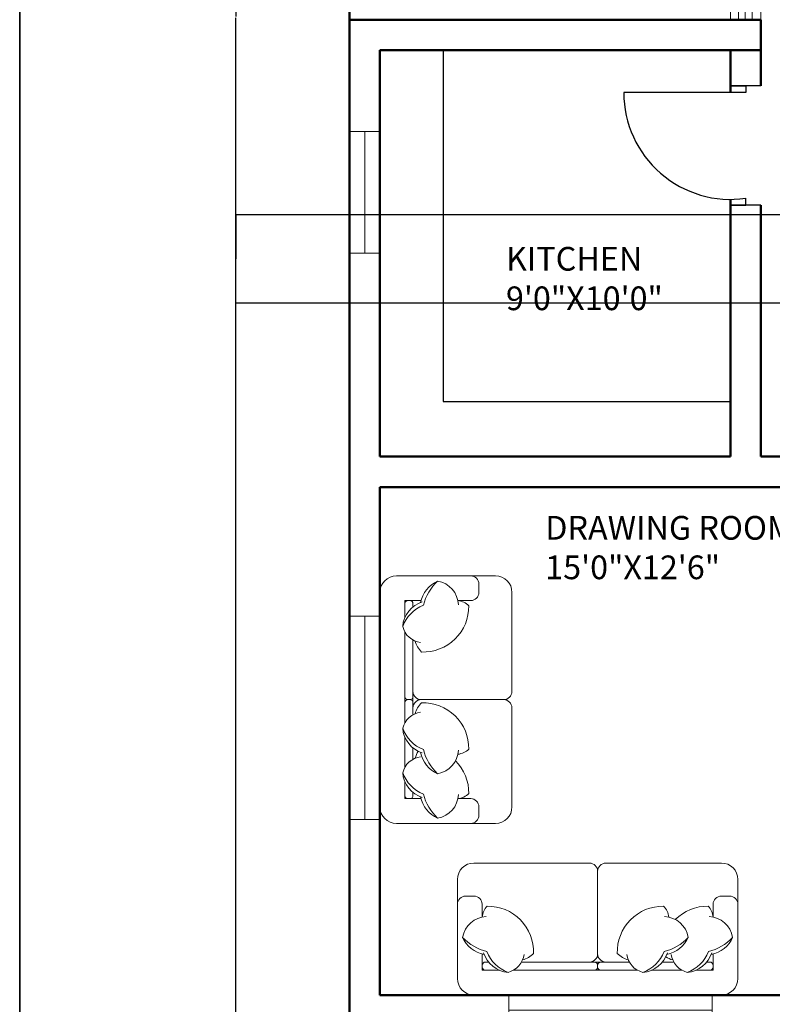
# Model space of a CAD drawing. Units: inches. Extents: x 2215 to 3724, y 1009 to 2124.
# Tile 2 of 11: x 2215 to 2438, y 1158 to 1449. Entities that reach past the tile are written whole.
import ezdxf

# ---------------------------------------------------------------- set-up
doc = ezdxf.new("R2010")
doc.units = ezdxf.units.IN
for name, color, linetype, lineweight in [('A-ANNO-DIMS', 2, 'Continuous', 18), ('A-ANNO-TTLB', 7, 'Continuous', 35), ('A-AREA-IDEN', 7, 'Continuous', 18), ('A-DOOR', 3, 'Continuous', 25), ('A-FLOR-CASE', 7, 'Continuous', 25), ('A-FURN', 8, 'Continuous', 18), ('A-GLAZ', 4, 'Continuous', 18), ('A-WALL', 7, 'Continuous', 50)]:
    doc.layers.add(name, color=color, linetype=linetype, lineweight=lineweight)
doc.styles.get("Standard").update_dxf_attribs({"font": 'arial.ttf'})
doc.dimstyles.get("Standard").update_dxf_attribs({"dimtxt": 0.18, "dimasz": 0.18, "dimexe": 0.18, "dimexo": 0.0625, "dimgap": 0.09, "dimtad": 0, "dimtih": 1, "dimtoh": 1, "dimdec": 4, "dimzin": 0, "dimdsep": 46, "dimtxsty": 'Standard', "dimcen": 0.09, "dimadec": 0, "dimazin": 0, "dimtfac": 1, "dimtdec": 4, "dimtofl": 0, "dimtmove": 0, "dimatfit": 3, "dimfxl": 1, "dimtolj": 1, "dimtzin": 0, "dimarcsym": 0})

# ---------------------------------------------------------------- blocks, each defined once
blk = doc.blocks.new('DOOR-KITCHEN')
for p, q in [((40.5, 35.21), (31.5, 35.21)), ((31.5, 35.21), (36, 35.21)), ((36, 35.21), (36, 33.21)), ((36, 33.21), (0, 33.21)), ((36, 0), (36, 2)), ((40.5, 0), (31.5, 0)), ((31.5, 0), (36, 0))]:
    blk.add_line(p, q)
blk.add_arc((31.53, 33.21), 31.53, 180, 278.1525)
blk = doc.blocks.new('WIN-60-JAMB-B')
for p, q in [((9, 60), (0, 60)), ((0, 60), (4.5, 60)), ((4.5, 60), (4.5, 0)), ((4.5, 0), (0, 0)), ((0, 0), (9, 0))]:
    blk.add_line(p, q)
blk = doc.blocks.new('SCREEN-LAUNDRY')
for p, q in [((0, 0), (0, 60)), ((0, 60), (9, 60)), ((4.37, 60), (2.37, 60)), ((2.37, 60), (2.37, 0)), ((4.37, 0), (4.37, 60)), ((6.37, 0), (6.37, 60)), ((9, 60), (9, 0)), ((2.37, 0), (4.37, 0)), ((9, 0), (4.37, 0)), ((4.37, 0), (6.37, 0))]:
    blk.add_line(p, q)
blk = doc.blocks.new('WIN-60-FRONT')
for p, q in [((0, 9), (0, 9)), ((0, 9), (0, 0)), ((60, 4.5), (60, 9)), ((60, 9), (60, 0)), ((0, 0), (0, 4.5)), ((0, 4.5), (60, 4.5))]:
    blk.add_line(p, q)
blk = doc.blocks.new('WIN-KITCHEN-36')
for p, q in [((0, 36), (9, 36)), ((9, 36), (4.5, 36)), ((4.5, 36), (4.5, 0)), ((4.5, 0), (0, 0)), ((0, 0), (9, 0))]:
    blk.add_line(p, q)
blk = doc.blocks.new('*D88')
at = {"layer": 'A-ANNO-DIMS', "color": 0, "lineweight": -2, "transparency": 16777216}
for p, q in [((2312.78, 1747.5), (2279.06, 1747.5)), ((2279.24, 1747.32), (2279.24, 1449.93)), ((2279.24, 1152.18), (2279.24, 1449.57)), ((2312.78, 1152), (2279.06, 1152))]:
    blk.add_line(p, q, dxfattribs=at)
at = {"layer": 'A-ANNO-DIMS', "color": 0, "transparency": 16777216}
for points in [[(2279.21, 1747.32), (2279.27, 1747.32), (2279.24, 1747.5)], [(2279.21, 1152.18), (2279.27, 1152.18), (2279.24, 1152)]]:
    blk.add_solid(points, dxfattribs=at)
at = {"layer": 'Defpoints', "color": 0, "transparency": 16777216}
for p in [(2279.24, 1747.5), (2312.84, 1747.5), (2312.84, 1152)]:
    blk.add_point(p, dxfattribs=at)
at = {"layer": 'A-ANNO-DIMS', "color": 0, "transparency": 16777216, "insert": (2279.24, 1449.75), "char_height": 0.18, "attachment_point": 5}
blk.add_mtext('\\A1;595.5', dxfattribs=at)
blk = doc.blocks.new('*D103')
at = {"layer": 'A-ANNO-DIMS', "color": 0, "lineweight": -2, "transparency": 16777216}
for p, q in [((2450.55, 1391.42), (2279.06, 1391.42)), ((2279.24, 1391.24), (2279.24, 1378.53)), ((2279.24, 1365.46), (2279.24, 1378.17)), ((2450.55, 1365.28), (2279.06, 1365.28))]:
    blk.add_line(p, q, dxfattribs=at)
at = {"layer": 'A-ANNO-DIMS', "color": 0, "transparency": 16777216}
for points in [[(2279.21, 1391.24), (2279.27, 1391.24), (2279.24, 1391.42)], [(2279.21, 1365.46), (2279.27, 1365.46), (2279.24, 1365.28)]]:
    blk.add_solid(points, dxfattribs=at)
at = {"layer": 'Defpoints', "color": 0, "transparency": 16777216}
for p in [(2279.24, 1391.42), (2450.62, 1391.42), (2450.62, 1365.28)]:
    blk.add_point(p, dxfattribs=at)
at = {"layer": 'A-ANNO-DIMS', "color": 0, "transparency": 16777216, "insert": (2279.24, 1378.35), "char_height": 0.18, "attachment_point": 5}
blk.add_mtext('\\A1;26.147', dxfattribs=at)

msp = doc.modelspace()

# ---------------------------------------------------------------- linework, layer by layer
at = {"layer": 'A-ANNO-TTLB'}
msp.add_lwpolyline([(2215.4438, 2124.2681), (3723.6589, 2124.2681), (3723.6589, 1008.7935), (2215.4438, 1008.7935)], close=True, dxfattribs=at)
at = {"layer": 'A-FLOR-CASE'}
for p, q in [((2340.5139, 1439.9969), (2340.5139, 1336.2381)), ((2340.5139, 1336.2381), (2425.341, 1336.2381))]:
    msp.add_line(p, q, dxfattribs=at)
at = {"layer": 'A-FURN', "ltscale": 0.03}
for points in [[(2360.8221, 1250.6567, -0.41421356), (2358.3857, 1248.2203, -0.41421356), (2360.8221, 1245.784), (2360.8221, 1216.5482, -0.41421356), (2355.9494, 1211.6756), (2326.7136, 1211.6756, -0.41421356), (2321.841, 1216.5482), (2321.841, 1279.8924, -0.41421356), (2326.7136, 1284.7651), (2355.9494, 1284.7651, -0.41421356), (2360.8221, 1279.8924), (2360.8221, 1250.6567, -0.41421356), (2358.3857, 1248.2203, -0.41421356), (2360.8221, 1245.784)], [(2383.6911, 1199.978, -0.41421356), (2386.1274, 1197.5417, -0.41421356), (2388.5637, 1199.978), (2422.6722, 1199.978, -0.41421356), (2427.5448, 1195.1054), (2427.5448, 1165.8696, -0.41421356), (2422.6722, 1160.9969), (2349.5827, 1160.9969, -0.41421356), (2344.71, 1165.8696), (2344.71, 1195.1054, -0.41421356), (2349.5827, 1199.978), (2383.6911, 1199.978, -0.41421356), (2386.1274, 1197.5417, -0.41421356), (2388.5637, 1199.978)]]:
    msp.add_lwpolyline(points, format="xyb", dxfattribs=at)
at = {"layer": 'A-FURN'}
for points in [[(2338.8722, 1283.2145, 0.14772988), (2334.6851, 1276.0939, 0.21334276), (2328.5441, 1269.8109, 0.17866181)], [(2345.0132, 1276.2335, 0.35677236), (2338.8722, 1283.2145, 0.24954205), (2333.8114, 1276.8891, -9.61688035)], [(2348.6405, 1284.7651, -0.41421356), (2351.0768, 1282.3288), (2351.0768, 1279.8924, -0.41421356), (2348.6405, 1277.4561), (2344.8657, 1277.4561)], [(2334.3514, 1277.0776, 0.30666349), (2328.5441, 1269.8109, 0.30632997), (2333.8477, 1265.0638, -0.87284716)], [(2331.5863, 1275.5969), (2331.5863, 1276.4816, 0.41421356), (2330.6117, 1277.4561), (2330.1245, 1277.4561, 0.41421356), (2329.1499, 1276.4816)], [(2329.1499, 1276.4816), (2329.1499, 1272.3308, 0.41421356)], [(2344.8646, 1277.4614, -0.16554063), (2348.0837, 1275.9542, -0.42598917), (2334.1268, 1262.2714, -0.12152332), (2332.2031, 1265.5195, 7.11546429)], [(2329.1499, 1268.2777), (2329.1499, 1249.1949, 0.41421356), (2330.1245, 1248.2203), (2330.6117, 1248.2203, 0.41421356), (2331.5863, 1249.1949), (2331.5863, 1265.8244, 0.41421356)], [(2331.5863, 1250.6567, 0.41421356), (2334.0226, 1248.2203)], [(2331.5863, 1250.6567, 0.41421356), (2334.0226, 1248.2203), (2358.3857, 1248.2203, 0.41421356)], [(2329.1499, 1241.2874), (2329.1499, 1247.2458, -0.41421356), (2330.1245, 1248.2203), (2330.6117, 1248.2203, -0.41421356), (2331.5863, 1247.2458), (2331.5863, 1243.7406, -0.41421356)], [(2331.5863, 1245.784, -0.41421356), (2334.0226, 1248.2203)], [(2331.5863, 1245.784, -0.41421356), (2334.0226, 1248.2203), (2358.3857, 1248.2203, -0.41421356)], [(2344.8646, 1232.1036, 0.16554063), (2348.0837, 1233.6108, 0.42598917), (2334.1268, 1247.2936, 0.12152332), (2332.2031, 1244.0455, -7.11546429)], [(2334.3514, 1232.4874, -0.30666349), (2328.5441, 1239.7541, -0.30632997), (2333.8477, 1244.5012, 0.87284716)], [(2338.8722, 1226.3505, -0.14772988), (2334.6851, 1233.4711, -0.21334276), (2328.5441, 1239.7541, -0.17866181)], [(2329.1499, 1228.163), (2329.1499, 1237.2342, -0.41421356)], [(2331.5863, 1233.9681), (2331.5863, 1230.6162, -0.41421356)], [(2333.1556, 1232.9638, 0.07186538), (2332.2031, 1230.9212, -7.11546429)], [(2345.0132, 1233.3315, -0.35677236), (2338.8722, 1226.3505, -0.24954205), (2333.8114, 1232.6759, 9.61688035)], [(2334.3514, 1219.3631, -0.30666349), (2328.5441, 1226.6297, -0.30632997), (2333.8477, 1231.3768, 0.87284716)], [(2344.8646, 1218.9792, 0.16554063), (2348.0837, 1220.4864, 0.20023115), (2344.1632, 1230.1577, 0.12152332)], [(2338.8722, 1213.2262, -0.14772988), (2334.6851, 1220.3468, -0.21334276), (2328.5441, 1226.6297, -0.17866181)], [(2329.1499, 1219.9591), (2329.1499, 1224.1099, -0.41421356)], [(2329.1499, 1224.1099), (2329.1499, 1218.9845), (2333.9379, 1218.9845, -0.41421356)], [(2331.5863, 1220.8437), (2331.5863, 1219.9591, -0.41421356), (2330.6117, 1218.9845), (2330.1245, 1218.9845, -0.41421356), (2329.1499, 1219.9591)], [(2345.0132, 1220.2072, -0.35677236), (2338.8722, 1213.2262, -0.24954205), (2333.8114, 1219.5516, 9.61688035)], [(2344.8657, 1218.9845), (2348.6405, 1218.9845, -0.41421356), (2351.0768, 1216.5482), (2351.0768, 1214.1119, -0.41421356), (2348.6405, 1211.6756)], [(2383.6911, 1170.7422, 0.41421356), (2386.1274, 1173.1785), (2386.1274, 1197.5417, 0.41421356)], [(2388.5637, 1170.7422, -0.41421356), (2386.1274, 1173.1785), (2386.1274, 1197.5417, -0.41421356)], [(2344.71, 1187.7964, -0.41421356), (2347.1463, 1190.2327), (2349.5827, 1190.2327, -0.41421356), (2352.019, 1187.7964), (2352.019, 1184.0217)], [(2420.2358, 1184.0217), (2420.2358, 1187.7964, -0.41421356), (2422.6722, 1190.2327), (2425.1085, 1190.2327, -0.41421356), (2427.5448, 1187.7964)], [(2352.0137, 1184.0206, -0.16554063), (2353.5209, 1187.2396, -0.42598917), (2367.2037, 1173.2828, -0.12152332), (2363.9556, 1171.3591, 7.11546429)], [(2407.1168, 1184.0206, 0.16554063), (2405.6096, 1187.2396, 0.42598917), (2391.9268, 1173.2828, 0.12152332), (2395.1748, 1171.3591, -7.11546429)], [(2420.2411, 1184.0206, 0.16554063), (2418.734, 1187.2396, 0.20023115), (2409.0627, 1183.3191, 0.12152332)], [(2353.2416, 1184.1691, 0.35677236), (2346.2606, 1178.0281, 0.24954205), (2352.586, 1172.9674, -9.61688035)], [(2405.8889, 1184.1691, -0.35677236), (2412.8699, 1178.0281, -0.24954205), (2406.5444, 1172.9674, 9.61688035)], [(2419.0132, 1184.1691, -0.35677236), (2425.9942, 1178.0281, -0.24954205), (2419.6688, 1172.9674, 9.61688035)], [(2346.2606, 1178.0281, 0.14772988), (2353.3812, 1173.8411, 0.21334276), (2359.6642, 1167.7, 0.17866181)], [(2412.8699, 1178.0281, -0.14772988), (2405.7492, 1173.8411, -0.21334276), (2399.4663, 1167.7, -0.17866181)], [(2425.9942, 1178.0281, -0.14772988), (2418.8736, 1173.8411, -0.21334276), (2412.5906, 1167.7, -0.17866181)], [(2352.3975, 1173.5074, 0.30666349), (2359.6642, 1167.7, 0.30632997), (2364.4113, 1173.0036, -0.87284716)], [(2383.6911, 1170.7422, 0.41421356), (2386.1274, 1173.1785)], [(2388.5637, 1170.7422, -0.41421356), (2386.1274, 1173.1785)], [(2406.733, 1173.5074, -0.30666349), (2399.4663, 1167.7, -0.30632997), (2394.7192, 1173.0036, 0.87284716)], [(2406.2566, 1172.3116, 0.07186538), (2408.2992, 1171.3591, -7.11546429)], [(2419.8573, 1173.5074, -0.30666349), (2412.5906, 1167.7, -0.30632997), (2407.8435, 1173.0036, 0.87284716)], [(2415.1105, 1168.3059), (2420.2358, 1168.3059), (2420.2358, 1173.0938, -0.41421356)], [(2353.8782, 1170.7422), (2352.9935, 1170.7422, 0.41421356), (2352.019, 1169.7677), (2352.019, 1169.2804, 0.41421356), (2352.9935, 1168.3059)], [(2361.1975, 1168.3059), (2385.1529, 1168.3059, 0.41421356), (2386.1274, 1169.2804), (2386.1274, 1169.7677, 0.41421356), (2385.1529, 1170.7422), (2363.6507, 1170.7422, 0.41421356)], [(2397.933, 1168.3059), (2387.1019, 1168.3059, -0.41421356), (2386.1274, 1169.2804), (2386.1274, 1169.7677, -0.41421356), (2387.1019, 1170.7422), (2395.4798, 1170.7422, -0.41421356)], [(2405.2523, 1170.7422), (2408.6041, 1170.7422, -0.41421356)], [(2418.3766, 1170.7422), (2419.2613, 1170.7422, -0.41421356), (2420.2358, 1169.7677), (2420.2358, 1169.2804, -0.41421356), (2419.2613, 1168.3059)], [(2352.9935, 1168.3059), (2357.1443, 1168.3059, 0.41421356)], [(2411.0574, 1168.3059), (2401.9862, 1168.3059, -0.41421356)], [(2419.2613, 1168.3059), (2415.1105, 1168.3059, -0.41421356)]]:
    msp.add_lwpolyline(points, format="xyb", dxfattribs=at)
for points in [[(2333.9379, 1277.4561), (2329.1499, 1277.4561), (2329.1499, 1272.3308)], [(2329.1499, 1268.2777), (2329.1499, 1241.2874)], [(2329.1499, 1237.2342), (2329.1499, 1228.163)], [(2352.019, 1173.0938), (2352.019, 1168.3059), (2357.1443, 1168.3059)], [(2361.1975, 1168.3059), (2397.933, 1168.3059)], [(2401.9862, 1168.3059), (2411.0574, 1168.3059)]]:
    msp.add_lwpolyline(points, dxfattribs=at)
for points in [[(2329.1499, 1249.1949), (2329.1499, 1247.2458, -0.41421356), (2330.1245, 1248.2203), (2330.6117, 1248.2203, -0.41421356), (2331.5863, 1247.2458), (2331.5863, 1249.1949, -0.41421356), (2330.6117, 1248.2203), (2330.1245, 1248.2203, -0.41421356)], [(2385.1529, 1168.3059), (2387.1019, 1168.3059, -0.41421356), (2386.1274, 1169.2804), (2386.1274, 1169.7677, -0.41421356), (2387.1019, 1170.7422), (2385.1529, 1170.7422, -0.41421356), (2386.1274, 1169.7677), (2386.1274, 1169.2804, -0.41421356)]]:
    msp.add_lwpolyline(points, format="xyb", close=True, dxfattribs=at)
at = {"layer": 'A-WALL'}
for p, q in [((2312.841, 1517.9969), (2312.841, 1151.9969)), ((2434.341, 1448.9969), (2312.841, 1448.9969)), ((2312.841, 1448.9969), (2425.341, 1448.9969)), ((2434.341, 1448.9969), (2434.341, 1429.4651)), ((2434.341, 1439.9969), (2321.841, 1439.9969)), ((2321.841, 1439.9969), (2321.841, 1319.9969)), ((2425.341, 1427.4651), (2425.341, 1439.9969)), ((2425.341, 1319.9969), (2425.341, 1395.9362)), ((2434.341, 1394.2548), (2434.341, 1319.9969)), ((2425.341, 1319.9969), (2321.841, 1319.9969)), ((2456.5044, 1319.9969), (2434.341, 1319.9969)), ((2321.841, 1310.9969), (2321.841, 1160.9969)), ((2458.7861, 1310.9969), (2321.841, 1310.9969)), ((2464.7699, 1160.9969), (2321.841, 1160.9969))]:
    msp.add_line(p, q, dxfattribs=at)

# ---------------------------------------------------------------- block references
at = {"layer": 'A-DOOR'}
msp.add_blockref('DOOR-KITCHEN', (2393.841, 1394.255), dxfattribs=at)
at = {"layer": 'A-GLAZ'}
for name, p in [('SCREEN-LAUNDRY', (2425.341, 1448.997)), ('WIN-KITCHEN-36', (2312.841, 1380.031)), ('WIN-60-JAMB-B', (2312.841, 1212.834)), ('WIN-60-FRONT', (2359.903, 1151.997))]:
    msp.add_blockref(name, p, dxfattribs=at)

# ---------------------------------------------------------------- texts
at = {"layer": 'A-AREA-IDEN', "char_height": 7, "attachment_point": 1}
for s, width, insert in [('KITCHEN\\P9\'0"X10\'0"', 144.730638, (2359.0447, 1381.8981)), ('DRAWING ROOM\\P15\'0"X12\'6"', 104.31309, (2370.6503, 1302.4617))]:
    msp.add_mtext_dynamic_manual_height_columns(s, width=width, gutter_width=12.5, heights=[0], dxfattribs=dict(at, insert=insert))

# ---------------------------------------------------------------- dimensions: what is measured, and where the dimension line sits
at = {"layer": 'A-ANNO-DIMS'}
for base, p1, p2, override, picture, middle in [((2279.241, 1747.4969), (2312.841, 1151.9969), (2312.841, 1747.4969), {"dimdec": 1, "dimlfac": 1, "dimrnd": 0, "dimzin": 0, "dimdsep": 46, "dimlunit": 2}, '*D88', (2279.241, 1449.7469)), ((2279.241, 1391.4229), (2450.6169, 1365.276), (2450.6169, 1391.4229), {"dimdec": 3, "dimlfac": 1, "dimrnd": 0, "dimzin": 0, "dimdsep": 46, "dimlunit": 2}, '*D103', (2279.241, 1378.3494))]:
    dim = msp.add_linear_dim(base=base, p1=p1, p2=p2, angle=90, dimstyle='Standard', override=override, dxfattribs=at)
    dim.commit()
    dim.dimension.update_dxf_attribs({"geometry": picture, "text_midpoint": middle})

doc.saveas('drawing.dxf')
